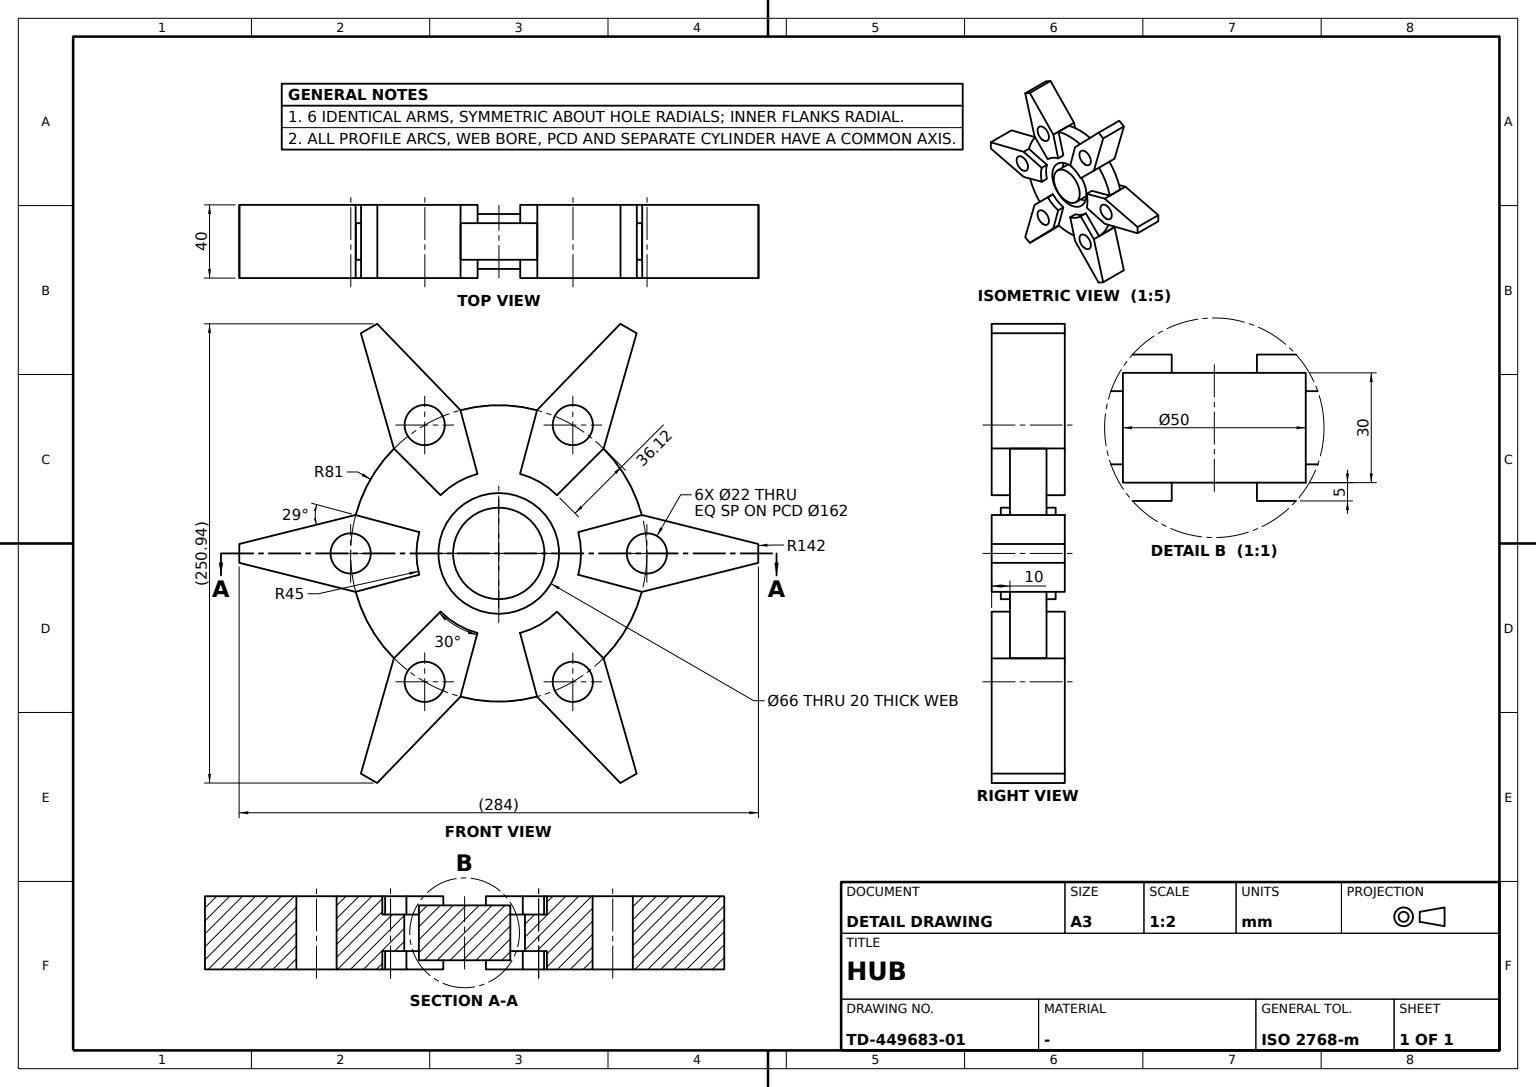
CATIA V5 part; units mm, degrees
sketch "Sketch1" plane through (0, 0, 0) normal (0, 0, 1) x (0, 1, 0)
  circle A0 centre (0, 0) radius 81
  dimension "radius A0" = 81
extrude "Pad1" add sketch "Sketch1" along normal mid plane 20
sketch "Sketch2" plane through (0, 0, 0) normal (0, 0, 1) x (0, 1, 0)
  arc A0 (43.4667, -11.6469) -> (43.4667, 11.6469) centre (0, 0) ccw
  line L0 (167.4153, 44.8588) -> (-170.6315, -45.7206) construction
  point P0 (167.4153, 44.8588)
  point P1 (-170.6315, -45.7206)
  point P2 (-170.6315, 45.7206)
  point P3 (167.4153, -44.8588)
  line L1 (167.4153, -44.8588) -> (-170.6315, 45.7206) construction
  line L2 (19.336, 35.712) -> (205.1106, -10.6067) construction
  point P4 (43.4667, 11.6469)
  line L3 (43.4667, 11.6469) -> (78.3585, 20.9961)
  point P5 (78.3585, 20.9961)
  line L4 (78.3585, 20.9961) -> (141.9065, 5.1518)
  point P6 (141.9065, 5.1518)
  point P7 (141.9065, -5.1518)
  point P8 (78.3585, -20.9961)
  line L5 (78.3585, -20.9961) -> (141.9065, -5.1518)
  point P9 (43.4667, -11.6469)
  line L6 (43.4667, -11.6469) -> (78.3585, -20.9961)
  point P10 (43.4667, -11.6469)
  point P11 (43.4667, 11.6469)
  arc A1 (141.9065, -5.1518) -> (141.9065, 5.1518) centre (0, 0) ccw
  point P12 (11.6469, 43.4667)
  point P13 (31.8198, 31.8198)
  arc A2 (31.8198, 31.8198) -> (11.6469, 43.4667) centre (0, 0) ccw
  point P14 (11.6469, 43.4667)
  line L7 (11.6469, 43.4667) -> (20.9961, 78.3585)
  line L8 (20.9961, 78.3585) -> (66.4917, 125.4705)
  point P15 (31.8198, 31.8198)
  line L9 (31.8198, 31.8198) -> (57.3624, 57.3624)
  line L10 (57.3624, 57.3624) -> (75.4148, 120.3187)
  arc A3 (75.4148, 120.3187) -> (66.4917, 125.4705) centre (0, 0) ccw
  point P16 (-31.8198, 31.8198)
  point P17 (-11.6469, 43.4667)
  arc A4 (-11.6469, 43.4667) -> (-31.8198, 31.8198) centre (0, 0) ccw
  point P18 (-31.8198, 31.8198)
  line L11 (-31.8198, 31.8198) -> (-57.3624, 57.3624)
  line L12 (-57.3624, 57.3624) -> (-75.4148, 120.3187)
  point P19 (-11.6469, 43.4667)
  line L13 (-11.6469, 43.4667) -> (-20.9961, 78.3585)
  line L14 (-20.9961, 78.3585) -> (-66.4917, 125.4705)
  arc A5 (-66.4917, 125.4705) -> (-75.4148, 120.3187) centre (0, 0) ccw
  point P20 (-43.4667, -11.6469)
  point P21 (-43.4667, 11.6469)
  arc A6 (-43.4667, 11.6469) -> (-43.4667, -11.6469) centre (0, 0) ccw
  point P22 (-43.4667, -11.6469)
  line L15 (-43.4667, -11.6469) -> (-78.3585, -20.9961)
  line L16 (-78.3585, -20.9961) -> (-141.9065, -5.1518)
  point P23 (-43.4667, 11.6469)
  line L17 (-43.4667, 11.6469) -> (-78.3585, 20.9961)
  line L18 (-78.3585, 20.9961) -> (-141.9065, 5.1518)
  arc A7 (-141.9065, 5.1518) -> (-141.9065, -5.1518) centre (0, 0) ccw
  point P24 (-11.6469, -43.4667)
  point P25 (-31.8198, -31.8198)
  arc A8 (-31.8198, -31.8198) -> (-11.6469, -43.4667) centre (0, 0) ccw
  point P26 (-11.6469, -43.4667)
  line L19 (-11.6469, -43.4667) -> (-20.9961, -78.3585)
  line L20 (-20.9961, -78.3585) -> (-66.4917, -125.4705)
  point P27 (-31.8198, -31.8198)
  line L21 (-31.8198, -31.8198) -> (-57.3624, -57.3624)
  line L22 (-57.3624, -57.3624) -> (-75.4148, -120.3187)
  arc A9 (-75.4148, -120.3187) -> (-66.4917, -125.4705) centre (0, 0) ccw
  point P28 (31.8198, -31.8198)
  point P29 (11.6469, -43.4667)
  arc A10 (11.6469, -43.4667) -> (31.8198, -31.8198) centre (0, 0) ccw
  point P30 (31.8198, -31.8198)
  line L23 (31.8198, -31.8198) -> (57.3624, -57.3624)
  line L24 (57.3624, -57.3624) -> (75.4148, -120.3187)
  point P31 (11.6469, -43.4667)
  line L25 (11.6469, -43.4667) -> (20.9961, -78.3585)
  line L26 (20.9961, -78.3585) -> (66.4917, -125.4705)
  arc A11 (66.4917, -125.4705) -> (75.4148, -120.3187) centre (0, 0) ccw
  dimension "radius A0" = 45
  dimension "angle x axis L0" = 15
  dimension "angle L2 L0" = 29
  constraint coincidence L0 origin
  constraint coincidence P4 A0
  constraint coincidence P4 L0
  constraint coincidence P5 L2
  constraint coincidence L1 P10
  constraint coincidence L0 P11
  constraint coincidence P4 P11
  constraint coincidence P9 P10
  constraint coincidence P12 P14
  constraint coincidence P13 P15
  constraint coincidence P16 P18
  constraint coincidence P17 P19
  constraint coincidence P20 P22
  constraint coincidence P21 P23
  constraint coincidence P24 P26
  constraint coincidence P25 P27
  constraint coincidence P28 P30
  constraint coincidence P29 P31
  constraint symmetry P1 P2 x-axis
  constraint symmetry P0 P3 x-axis
  constraint symmetry L0 L1 x-axis
  constraint symmetry P6 P7 x-axis
  constraint symmetry P5 P8 x-axis
  constraint symmetry L4 L5 x-axis
  constraint symmetry P4 P9 x-axis
  constraint symmetry L3 L6 x-axis
  constraint parallelism L3 L0
  constraint parallelism L4 L2
extrude "Pad2" add sketch "Sketch2" along normal mid plane 40
sketch "Sketch3" plane through (0, 0, 0) normal (0, 0, 1) x (0, 1, 0)
  circle A0 centre (81, 0) radius 11
  point P0 (81, 0)
  circle A1 centre (40.5, 70.1481) radius 11
  circle A2 centre (-40.5, 70.1481) radius 11
  circle A3 centre (-81, 0) radius 11
  circle A4 centre (-40.5, -70.1481) radius 11
  circle A5 centre (40.5, -70.1481) radius 11
  dimension "radius A0" = 11
  dimension "distance origin P0" = 81
  constraint coincidence P0 x-axis
extrude "Pocket1" cut sketch "Sketch3" along normal mid plane 40
sketch "Sketch4" plane through (0, 0, 0) normal (0, 0, 1) x (0, 1, 0)
  circle A0 centre (0, 0) radius 33
  dimension "radius A0" = 33
extrude "Pocket2" cut sketch "Sketch4" along normal mid plane 30
sketch "Sketch5" plane through (0, 0, 0) normal (0, 0, 1) x (1, 0, 0)
  circle A0 centre (0, 0) radius 25
  dimension "radius A0" = 25
extrude "Pad3" add sketch "Sketch5" along normal mid plane 30
